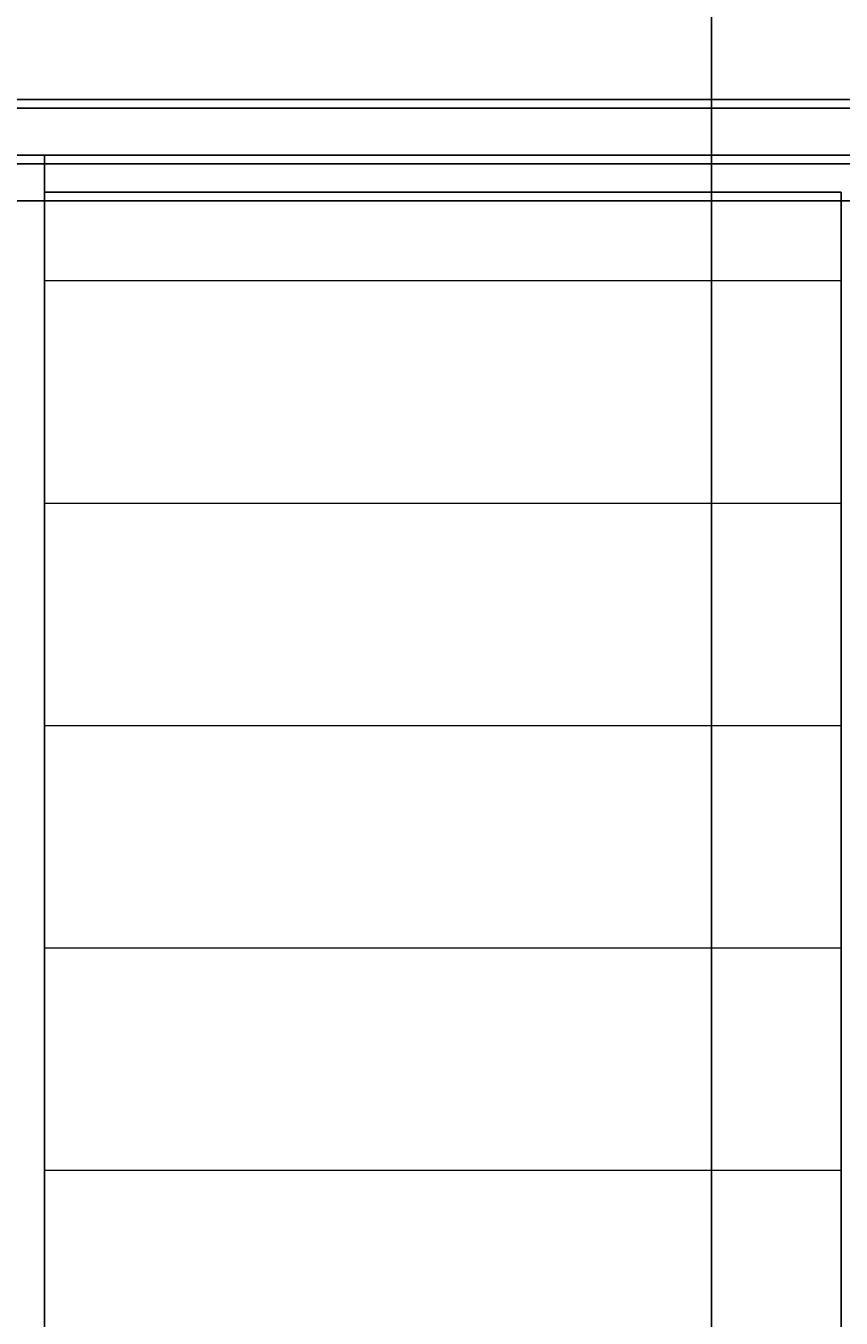
# Model space of a CAD drawing. Units: inches. Extents: x -6 to 289, y -8 to 323.
# Tile 71 of 107: x 212 to 234, y 194 to 229. Entities that reach past the tile are written whole.
import ezdxf

# ---------------------------------------------------------------- set-up
doc = ezdxf.new("R2010")
doc.units = ezdxf.units.IN
doc.header["$MEASUREMENT"] = 0
for name, color, linetype, lineweight in [('A-ANNO-DIMS', 2, 'Continuous', 18), ('A-ELEV-PATT', 8, 'Continuous', 13), ('A-GLAZ', 4, 'Continuous', 25)]:
    doc.layers.add(name, color=color, linetype=linetype, lineweight=lineweight)
doc.styles.get("Standard").update_dxf_attribs({"font": 'arial.ttf'})
doc.dimstyles.get("Standard").update_dxf_attribs({"dimtxt": 0.18, "dimasz": 0.18, "dimexe": 0.18, "dimexo": 0.0625, "dimgap": 0.09, "dimtad": 0, "dimtih": 1, "dimtoh": 1, "dimdec": 4, "dimzin": 0, "dimdsep": 46, "dimtxsty": 'Standard', "dimcen": 0.09, "dimadec": 0, "dimazin": 0, "dimtfac": 1, "dimtdec": 4, "dimtofl": 0, "dimtmove": 0, "dimatfit": 3, "dimfxl": 1, "dimtolj": 1, "dimtzin": 0, "dimarcsym": 0})

# ---------------------------------------------------------------- blocks, each defined once
blk = doc.blocks.new('*D13')
at = {"layer": 'A-ANNO-DIMS', "color": 0, "lineweight": -2, "transparency": 16777216}
for p, q in [((188.292, 226.951), (188.292, 322.969)), ((236.292, 226.951), (236.292, 322.969)), ((188.472, 322.789), (212.069, 322.789)), ((236.112, 322.789), (212.515, 322.789))]:
    blk.add_line(p, q, dxfattribs=at)
at = {"layer": 'A-ANNO-DIMS', "color": 0, "transparency": 16777216}
for points in [[(188.472, 322.819), (188.472, 322.759), (188.292, 322.789)], [(236.112, 322.819), (236.112, 322.759), (236.292, 322.789)]]:
    blk.add_solid(points, dxfattribs=at)
at = {"layer": 'Defpoints', "color": 0, "transparency": 16777216}
for p in [(236.292, 322.789), (188.292, 226.889), (236.292, 226.889)]:
    blk.add_point(p, dxfattribs=at)
at = {"layer": 'A-ANNO-DIMS', "color": 0, "transparency": 16777216, "insert": (212.292, 322.789), "char_height": 0.18, "attachment_point": 5}
blk.add_mtext('\\A1;48', dxfattribs=at)
blk = doc.blocks.new('*D25')
at = {"layer": 'A-ANNO-DIMS', "color": 0, "lineweight": -2, "transparency": 16777216}
for p, q in [((126.946, 226.654), (288.653, 226.654)), ((288.473, 226.474), (288.473, 202.836)), ((288.473, 178.834), (288.473, 202.472)), ((126.946, 178.654), (288.653, 178.654))]:
    blk.add_line(p, q, dxfattribs=at)
at = {"layer": 'A-ANNO-DIMS', "color": 0, "transparency": 16777216}
for points in [[(288.443, 226.474), (288.503, 226.474), (288.473, 226.654)], [(288.443, 178.834), (288.503, 178.834), (288.473, 178.654)]]:
    blk.add_solid(points, dxfattribs=at)
at = {"layer": 'Defpoints', "color": 0, "transparency": 16777216}
for p in [(126.883, 226.654), (288.473, 226.654), (126.883, 178.654)]:
    blk.add_point(p, dxfattribs=at)
at = {"layer": 'A-ANNO-DIMS', "color": 0, "transparency": 16777216, "insert": (288.473, 202.654), "char_height": 0.18, "attachment_point": 5}
blk.add_mtext('\\A1;48', dxfattribs=at)
blk = doc.blocks.new('*D26')
at = {"layer": 'A-ANNO-DIMS', "color": 0, "lineweight": -2, "transparency": 16777216}
for p, q in [((247.226, 247.289), (288.653, 247.289)), ((288.473, 247.109), (288.473, 237.153)), ((288.473, 226.834), (288.473, 236.789)), ((126.946, 226.654), (288.653, 226.654))]:
    blk.add_line(p, q, dxfattribs=at)
at = {"layer": 'A-ANNO-DIMS', "color": 0, "transparency": 16777216}
for points in [[(288.443, 247.109), (288.503, 247.109), (288.473, 247.289)], [(288.443, 226.834), (288.503, 226.834), (288.473, 226.654)]]:
    blk.add_solid(points, dxfattribs=at)
at = {"layer": 'Defpoints', "color": 0, "transparency": 16777216}
for p in [(247.164, 247.289), (288.473, 247.289), (126.883, 226.654)]:
    blk.add_point(p, dxfattribs=at)
at = {"layer": 'A-ANNO-DIMS', "color": 0, "transparency": 16777216, "insert": (288.473, 236.971), "char_height": 0.18, "attachment_point": 5}
blk.add_mtext('\\A1;20.635', dxfattribs=at)
blk = doc.blocks.new('*D37')
at = {"layer": 'A-ANNO-DIMS', "color": 0, "lineweight": -2, "transparency": 16777216}
for p, q in [((166.446, 224.154), (288.653, 224.154)), ((288.473, 223.974), (288.473, 202.836)), ((288.473, 181.334), (288.473, 202.472)), ((166.446, 181.154), (288.653, 181.154))]:
    blk.add_line(p, q, dxfattribs=at)
at = {"layer": 'A-ANNO-DIMS', "color": 0, "transparency": 16777216}
for points in [[(288.443, 223.974), (288.503, 223.974), (288.473, 224.154)], [(288.443, 181.334), (288.503, 181.334), (288.473, 181.154)]]:
    blk.add_solid(points, dxfattribs=at)
at = {"layer": 'Defpoints', "color": 0, "transparency": 16777216}
for p in [(166.383, 224.154), (288.473, 224.154), (166.383, 181.154)]:
    blk.add_point(p, dxfattribs=at)
at = {"layer": 'A-ANNO-DIMS', "color": 0, "transparency": 16777216, "insert": (288.473, 202.654), "char_height": 0.18, "attachment_point": 5}
blk.add_mtext('\\A1;43', dxfattribs=at)
blk = doc.blocks.new('*D38')
at = {"layer": 'A-ANNO-DIMS', "color": 0, "lineweight": -2, "transparency": 16777216}
for p, q in [((167.446, 225.154), (288.653, 225.154)), ((288.473, 224.974), (288.473, 224.834)), ((288.473, 224.334), (288.473, 224.474)), ((166.446, 224.154), (288.653, 224.154))]:
    blk.add_line(p, q, dxfattribs=at)
at = {"layer": 'A-ANNO-DIMS', "color": 0, "transparency": 16777216}
for points in [[(288.443, 224.974), (288.503, 224.974), (288.473, 225.154)], [(288.443, 224.334), (288.503, 224.334), (288.473, 224.154)]]:
    blk.add_solid(points, dxfattribs=at)
at = {"layer": 'Defpoints', "color": 0, "transparency": 16777216}
for p in [(167.383, 225.154), (288.473, 225.154), (166.383, 224.154)]:
    blk.add_point(p, dxfattribs=at)
at = {"layer": 'A-ANNO-DIMS', "color": 0, "transparency": 16777216, "insert": (288.473, 224.654), "char_height": 0.18, "attachment_point": 5}
blk.add_mtext('\\A1;1', dxfattribs=at)
blk = doc.blocks.new('*D39')
at = {"layer": 'A-ANNO-DIMS', "color": 0, "lineweight": -2, "transparency": 16777216}
for p, q in [((168.946, 226.654), (288.653, 226.654)), ((288.473, 226.474), (288.473, 226.086)), ((288.473, 225.334), (288.473, 225.722)), ((167.446, 225.154), (288.653, 225.154))]:
    blk.add_line(p, q, dxfattribs=at)
at = {"layer": 'A-ANNO-DIMS', "color": 0, "transparency": 16777216}
for points in [[(288.443, 226.474), (288.503, 226.474), (288.473, 226.654)], [(288.443, 225.334), (288.503, 225.334), (288.473, 225.154)]]:
    blk.add_solid(points, dxfattribs=at)
at = {"layer": 'Defpoints', "color": 0, "transparency": 16777216}
for p in [(168.883, 226.654), (288.473, 226.654), (167.383, 225.154)]:
    blk.add_point(p, dxfattribs=at)
at = {"layer": 'A-ANNO-DIMS', "color": 0, "transparency": 16777216, "insert": (288.473, 225.904), "char_height": 0.18, "attachment_point": 5}
blk.add_mtext('\\A1;1.5', dxfattribs=at)
blk = doc.blocks.new('*D43')
at = {"layer": 'A-ANNO-DIMS', "color": 0, "lineweight": -2, "transparency": 16777216}
for p, q in [((211.292, 224.326), (211.292, -8.391)), ((212.292, 224.326), (212.292, -8.391)), ((211.472, -8.211), (211.669, -8.211)), ((212.112, -8.211), (211.915, -8.211))]:
    blk.add_line(p, q, dxfattribs=at)
at = {"layer": 'A-ANNO-DIMS', "color": 0, "transparency": 16777216}
for points in [[(211.472, -8.181), (211.472, -8.241), (211.292, -8.211)], [(212.112, -8.181), (212.112, -8.241), (212.292, -8.211)]]:
    blk.add_solid(points, dxfattribs=at)
at = {"layer": 'Defpoints', "color": 0, "transparency": 16777216}
for p in [(211.292, 224.389), (212.292, 224.389), (212.292, -8.211)]:
    blk.add_point(p, dxfattribs=at)
at = {"layer": 'A-ANNO-DIMS', "color": 0, "transparency": 16777216, "insert": (211.792, -8.211), "char_height": 0.18, "attachment_point": 5}
blk.add_mtext('\\A1;1', dxfattribs=at)
blk = doc.blocks.new('*D44')
at = {"layer": 'A-ANNO-DIMS', "color": 0, "lineweight": -2, "transparency": 16777216}
for p, q in [((212.292, 224.326), (212.292, -8.391)), ((233.792, 224.326), (233.792, -8.391)), ((212.472, -8.211), (222.716, -8.211)), ((233.612, -8.211), (223.368, -8.211))]:
    blk.add_line(p, q, dxfattribs=at)
at = {"layer": 'A-ANNO-DIMS', "color": 0, "transparency": 16777216}
for points in [[(212.472, -8.181), (212.472, -8.241), (212.292, -8.211)], [(233.612, -8.181), (233.612, -8.241), (233.792, -8.211)]]:
    blk.add_solid(points, dxfattribs=at)
at = {"layer": 'Defpoints', "color": 0, "transparency": 16777216}
for p in [(212.292, 224.389), (233.792, 224.389), (233.792, -8.211)]:
    blk.add_point(p, dxfattribs=at)
at = {"layer": 'A-ANNO-DIMS', "color": 0, "transparency": 16777216, "insert": (223.042, -8.211), "char_height": 0.18, "attachment_point": 5}
blk.add_mtext('\\A1;21.5', dxfattribs=at)
blk = doc.blocks.new('*D80')
at = {"layer": 'A-ANNO-DIMS', "color": 0, "lineweight": -2, "transparency": 16777216}
for p, q in [((188.292, 116.842), (188.292, 322.969)), ((230.292, 116.842), (230.292, 322.969)), ((188.472, 322.789), (209.07, 322.789)), ((230.112, 322.789), (209.513, 322.789))]:
    blk.add_line(p, q, dxfattribs=at)
at = {"layer": 'A-ANNO-DIMS', "color": 0, "transparency": 16777216}
for points in [[(188.472, 322.819), (188.472, 322.759), (188.292, 322.789)], [(230.112, 322.819), (230.112, 322.759), (230.292, 322.789)]]:
    blk.add_solid(points, dxfattribs=at)
at = {"layer": 'Defpoints', "color": 0, "transparency": 16777216}
for p in [(230.292, 322.789), (188.292, 116.779), (230.292, 116.779)]:
    blk.add_point(p, dxfattribs=at)
at = {"layer": 'A-ANNO-DIMS', "color": 0, "transparency": 16777216, "insert": (209.292, 322.789), "char_height": 0.18, "attachment_point": 5}
blk.add_mtext('\\A1;42', dxfattribs=at)
blk = doc.blocks.new('*D81')
at = {"layer": 'A-ANNO-DIMS', "color": 0, "lineweight": -2, "transparency": 16777216}
for p, q in [((230.292, 68.842), (230.292, 322.969)), ((245.215, 66.286), (245.215, 322.969)), ((230.472, 322.789), (237.298, 322.789)), ((245.035, 322.789), (238.208, 322.789))]:
    blk.add_line(p, q, dxfattribs=at)
at = {"layer": 'A-ANNO-DIMS', "color": 0, "transparency": 16777216}
for points in [[(230.472, 322.819), (230.472, 322.759), (230.292, 322.789)], [(245.035, 322.819), (245.035, 322.759), (245.215, 322.789)]]:
    blk.add_solid(points, dxfattribs=at)
at = {"layer": 'Defpoints', "color": 0, "transparency": 16777216}
for p in [(245.215, 322.789), (230.292, 68.779), (245.215, 66.224)]:
    blk.add_point(p, dxfattribs=at)
at = {"layer": 'A-ANNO-DIMS', "color": 0, "transparency": 16777216, "insert": (237.753, 322.789), "char_height": 0.18, "attachment_point": 5}
blk.add_mtext('\\A1;14.923', dxfattribs=at)
blk = doc.blocks.new('*D98')
at = {"layer": 'A-ANNO-DIMS', "color": 0, "lineweight": -2, "transparency": 16777216}
for p, q in [((202.741, 159.411), (202.741, 322.969)), ((244.164, 159.411), (244.164, 322.969)), ((202.921, 322.789), (223.056, 322.789)), ((243.984, 322.789), (223.849, 322.789))]:
    blk.add_line(p, q, dxfattribs=at)
at = {"layer": 'A-ANNO-DIMS', "color": 0, "transparency": 16777216}
for points in [[(202.921, 322.819), (202.921, 322.759), (202.741, 322.789)], [(243.984, 322.819), (243.984, 322.759), (244.164, 322.789)]]:
    blk.add_solid(points, dxfattribs=at)
at = {"layer": 'Defpoints', "color": 0, "transparency": 16777216}
for p in [(244.164, 322.789), (202.741, 159.348), (244.164, 159.348)]:
    blk.add_point(p, dxfattribs=at)
at = {"layer": 'A-ANNO-DIMS', "color": 0, "transparency": 16777216, "insert": (223.452, 322.789), "char_height": 0.18, "attachment_point": 5}
blk.add_mtext('\\A1;41.42', dxfattribs=at)

msp = doc.modelspace()

# ---------------------------------------------------------------- hatches: boundary and pattern name
at = {"layer": 'A-ELEV-PATT'}
h = msp.add_hatch(dxfattribs=at)
h.set_pattern_fill('_USER', color=256, scale=6, pattern_type=0)
h.set_pattern_definition([(0, (0, 0), (0, 6), [])])
h.paths.add_polyline_path([(184.1244, 48.0851), (124.008, 48.0851), (124.008, 10.2888), (184.1244, 10.2888)])
h.paths.add_polyline_path([(244.2408, 48.0851), (186.3604, 48.0851), (186.3604, 10.2888), (244.2408, 10.2888)])
h.paths.add_polyline_path([(208.2918, 114.2795), (190.7918, 114.2795), (190.7918, 71.2795), (208.2918, 71.2795)])
h.paths.add_polyline_path([(227.7918, 114.2795), (209.2918, 114.2795), (209.2918, 71.2795), (227.7918, 71.2795)])
h.paths.add_polyline_path([(211.2918, 224.3887), (190.7918, 224.3887), (190.7918, 162.3484), (211.2918, 162.3484)])
h.paths.add_polyline_path([(233.7918, 224.3887), (212.2918, 224.3887), (212.2918, 162.3484), (233.7918, 162.3484)])
h.paths.add_polyline_path([(166.3835, 224.154), (147.8835, 224.154), (147.8835, 181.154), (166.3835, 181.154)])
h.paths.add_polyline_path([(146.8835, 224.154), (129.3835, 224.154), (129.3835, 181.154), (146.8835, 181.154)])

# ---------------------------------------------------------------- linework, layer by layer
at = {"layer": 'A-GLAZ'}
for p, q in [((189.7918, 225.3887), (212.2918, 225.3887)), ((212.2918, 225.3887), (234.7918, 225.3887)), ((212.2918, 162.3484), (212.2918, 225.3887))]:
    msp.add_line(p, q, dxfattribs=at)
for points in [[(188.2918, 162.3484), (188.2918, 226.8887), (236.2918, 226.8887), (236.2918, 162.3484)], [(212.2918, 224.3887), (233.7918, 224.3887), (233.7918, 162.3484)]]:
    msp.add_lwpolyline(points, dxfattribs=at)

# ---------------------------------------------------------------- dimensions: what is measured, and where the dimension line sits
at = {"layer": 'A-ANNO-DIMS'}
for base, p1, p2, override, picture, middle in [((236.2918, 322.7888), (188.2918, 226.8887), (236.2918, 226.8887), {"dimdec": 0, "dimlfac": 1, "dimrnd": 0, "dimzin": 0, "dimdsep": 46, "dimlunit": 2}, '*D13', (212.2918, 322.7888)), ((230.2918, 322.7888), (188.2918, 116.7795), (230.2918, 116.7795), {"dimdec": 0, "dimlfac": 1, "dimrnd": 0, "dimzin": 0, "dimdsep": 46, "dimlunit": 2}, '*D80', (209.2918, 322.7888)), ((244.1638, 322.7888), (202.741, 159.3484), (244.1638, 159.3484), {"dimdec": 2, "dimlfac": 1, "dimrnd": 0, "dimzin": 0, "dimdsep": 46, "dimlunit": 2}, '*D98', (223.4524, 322.7888)), ((245.2146, 322.7888), (230.2918, 68.7795), (245.2146, 66.2238), {"dimdec": 3, "dimlfac": 1, "dimrnd": 0, "dimzin": 0, "dimdsep": 46, "dimlunit": 2}, '*D81', (237.7532, 322.7888)), ((212.2918, -8.2112), (211.2918, 224.3887), (212.2918, 224.3887), {"dimdec": 0, "dimlfac": 1, "dimrnd": 0, "dimzin": 0, "dimdsep": 46, "dimlunit": 2}, '*D43', (211.7918, -8.2112)), ((233.7918, -8.2112), (212.2918, 224.3887), (233.7918, 224.3887), {"dimdec": 1, "dimlfac": 1, "dimrnd": 0, "dimzin": 0, "dimdsep": 46, "dimlunit": 2}, '*D44', (223.0418, -8.2112))]:
    dim = msp.add_linear_dim(base=base, p1=p1, p2=p2, dimstyle='Standard', override=override, dxfattribs=at)
    dim.commit()
    dim.dimension.update_dxf_attribs({"geometry": picture, "text_midpoint": middle})
for base, p1, p2, override, picture, middle in [((288.4733, 247.2888), (126.8835, 226.654), (247.1638, 247.2888), {"dimdec": 3, "dimlfac": 1, "dimrnd": 0, "dimzin": 0, "dimdsep": 46, "dimlunit": 2}, '*D26', (288.4733, 236.9714)), ((288.4733, 226.654), (126.8835, 178.654), (126.8835, 226.654), {"dimdec": 0, "dimlfac": 1, "dimrnd": 0, "dimzin": 0, "dimdsep": 46, "dimlunit": 2}, '*D25', (288.4733, 202.654)), ((288.4733, 226.654), (167.3835, 225.154), (168.8835, 226.654), {"dimdec": 1, "dimlfac": 1, "dimrnd": 0, "dimzin": 0, "dimdsep": 46, "dimlunit": 2}, '*D39', (288.4733, 225.904)), ((288.4733, 225.154), (166.3835, 224.154), (167.3835, 225.154), {"dimdec": 0, "dimlfac": 1, "dimrnd": 0, "dimzin": 0, "dimdsep": 46, "dimlunit": 2}, '*D38', (288.4733, 224.654)), ((288.4733, 224.154), (166.3835, 181.154), (166.3835, 224.154), {"dimdec": 0, "dimlfac": 1, "dimrnd": 0, "dimzin": 0, "dimdsep": 46, "dimlunit": 2}, '*D37', (288.4733, 202.654))]:
    dim = msp.add_linear_dim(base=base, p1=p1, p2=p2, angle=90, dimstyle='Standard', override=override, dxfattribs=at)
    dim.commit()
    dim.dimension.update_dxf_attribs({"geometry": picture, "text_midpoint": middle})

doc.saveas('drawing.dxf')
